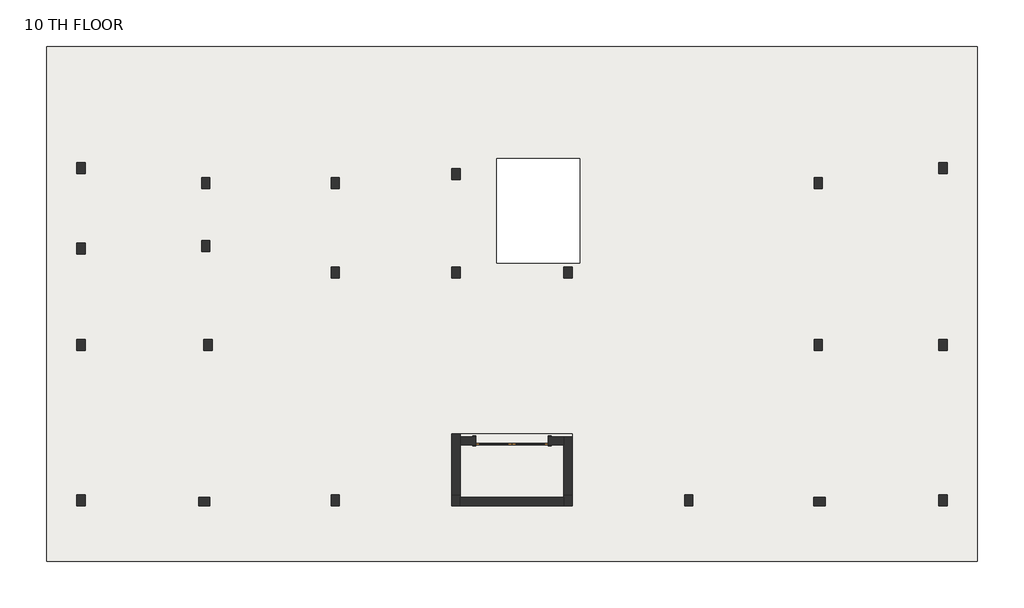
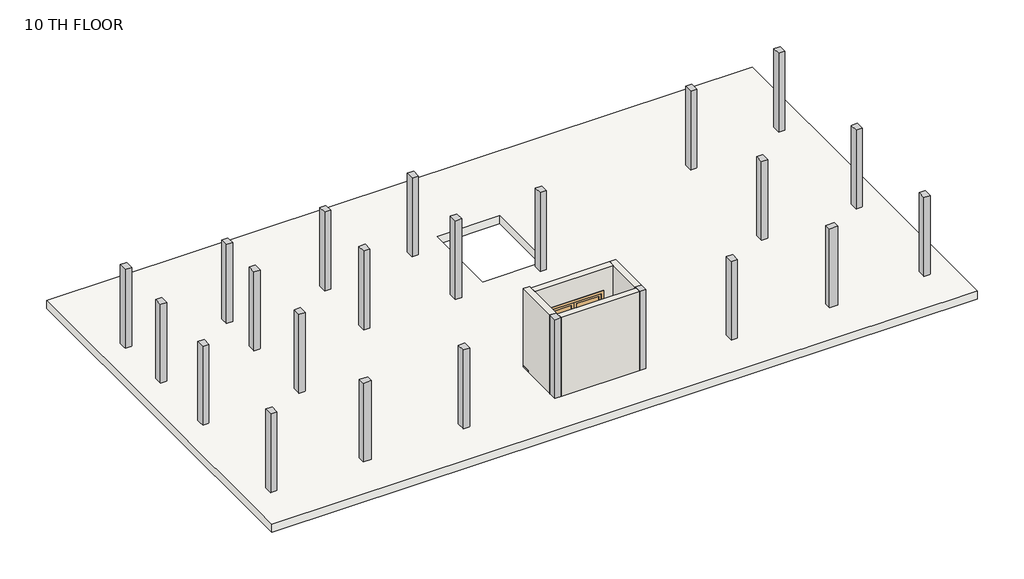
# One storey: 23 columns, 4 walls, 2 slabs, 1 door.
"""IFC4 building model written with IfcOpenShell, lengths in millimetres."""

from ifc_helpers import new_model, si_unit, frame, origin, place, context, project, spatial, polyline, outline, extrude, faceted_brep, transform, mapped, element, save
from components import column_69e4a381, door_77e2dd85

model = new_model("IFC4")

# Units and contexts
model_context = context("Model", 3, world=origin())
ifc_project = project(units=[si_unit("LENGTHUNIT", "METRE", prefix="MILLI")], contexts=[model_context])

# Site, building, storey
site = spatial("IfcSite", under=ifc_project)
building = spatial("IfcBuilding", under=site)
storey = spatial("IfcBuildingStorey", under=building, Name="10 TH FLOOR", Elevation=35204.4)

# Columns
placement = place(None, origin())
element("IfcColumn", 1, ObjectType="Rectangular Column : 1'X 9\"", at=placement, inside=storey, context=model_context, shape_type="SweptSolid", body=[
    extrude(outline(polyline([(-12224.6987957, -3709.2932671), (-12224.6987957, -4014.0932671), (-12453.2987957, -4014.0932671), (-12453.2987957, -3709.2932671), (-12224.6987957, -3709.2932671)])), frame((0.0, 0.0, 35204.4), z_axis=(0.0, 0.0, 1.0), x_axis=(1.0, 0.0, 0.0)), (0.0, 0.0, 1.0), 3048.0),
])
element("IfcColumn", 2, ObjectType="Rectangular Column : 1'X 9\"", at=placement, inside=storey, context=model_context, shape_type="SweptSolid", body=[
    extrude(outline(polyline([(-12224.6987957, 583.3067334), (-12224.6987957, 278.5067334), (-12453.2987957, 278.5067334), (-12453.2987957, 583.3067334), (-12224.6987957, 583.3067334)])), frame((0.0, 0.0, 35204.4), z_axis=(0.0, 0.0, 1.0), x_axis=(1.0, 0.0, 0.0)), (0.0, 0.0, 1.0), 3048.0),
])
element("IfcColumn", 3, ObjectType="Rectangular Column : 1'X 9\"", at=placement, inside=storey, context=model_context, shape_type="SweptSolid", body=[
    extrude(outline(polyline([(-12224.6987957, 3256.6567332), (-12224.6987957, 2951.8567332), (-12453.2987957, 2951.8567332), (-12453.2987957, 3256.6567332), (-12224.6987957, 3256.6567332)])), frame((0.0, 0.0, 35204.4), z_axis=(0.0, 0.0, 1.0), x_axis=(1.0, 0.0, 0.0)), (0.0, 0.0, 1.0), 3048.0),
])
element("IfcColumn", 4, ObjectType="Rectangular Column : 1'X 9\"", at=placement, inside=storey, context=model_context, shape_type="SweptSolid", body=[
    extrude(outline(polyline([(-8770.2987992, 5066.406733), (-8770.2987992, 4761.606733), (-8998.8987992, 4761.606733), (-8998.8987992, 5066.406733), (-8770.2987992, 5066.406733)])), frame((0.0, 0.0, 35204.4), z_axis=(0.0, 0.0, 1.0), x_axis=(1.0, 0.0, 0.0)), (0.0, 0.0, 1.0), 3048.0),
])
element("IfcColumn", 5, ObjectType="Rectangular Column : 1'X 9\"", at=placement, inside=storey, context=model_context, shape_type="SweptSolid", body=[
    extrude(outline(polyline([(-8770.2987992, 3326.5067332), (-8770.2987992, 3021.7067332), (-8998.8987992, 3021.7067332), (-8998.8987992, 3326.5067332), (-8770.2987992, 3326.5067332)])), frame((0.0, 0.0, 35204.4), z_axis=(0.0, 0.0, 1.0), x_axis=(1.0, 0.0, 0.0)), (0.0, 0.0, 1.0), 3048.0),
])
element("IfcColumn", 6, ObjectType="Rectangular Column : 1'X 9\"", at=placement, inside=storey, context=model_context, shape_type="SweptSolid", body=[
    extrude(outline(polyline([(-8713.148796, 583.3067334), (-8713.148796, 278.5067334), (-8941.748796, 278.5067334), (-8941.748796, 583.3067334), (-8713.148796, 583.3067334)])), frame((0.0, 0.0, 35204.4), z_axis=(0.0, 0.0, 1.0), x_axis=(1.0, 0.0, 0.0)), (0.0, 0.0, 1.0), 3048.0),
])
element("IfcColumn", 7, ObjectType="Rectangular Column : 1'X 9\"", at=placement, inside=storey, context=model_context, shape_type="SweptSolid", body=[
    extrude(outline(polyline([(-5188.8987995, 5066.406733), (-5188.8987995, 4761.606733), (-5417.4987995, 4761.606733), (-5417.4987995, 5066.406733), (-5188.8987995, 5066.406733)])), frame((0.0, 0.0, 35204.4), z_axis=(0.0, 0.0, 1.0), x_axis=(1.0, 0.0, 0.0)), (0.0, 0.0, 1.0), 3048.0),
])
element("IfcColumn", 8, ObjectType="Rectangular Column : 1'X 9\"", at=placement, inside=storey, context=model_context, shape_type="SweptSolid", body=[
    extrude(outline(polyline([(-5188.8987995, 2589.9067802), (-5188.8987995, 2285.1067802), (-5417.4987995, 2285.1067802), (-5417.4987995, 2589.9067802), (-5188.8987995, 2589.9067802)])), frame((0.0, 0.0, 35204.4), z_axis=(0.0, 0.0, 1.0), x_axis=(1.0, 0.0, 0.0)), (0.0, 0.0, 1.0), 3048.0),
])
element("IfcColumn", 9, ObjectType="Rectangular Column : 1'X 9\"", at=placement, inside=storey, context=model_context, shape_type="SweptSolid", body=[
    extrude(outline(polyline([(-5188.8987963, -3709.2932193), (-5188.8987963, -4014.0932193), (-5417.4987963, -4014.0932193), (-5417.4987963, -3709.2932193), (-5188.8987963, -3709.2932193)])), frame((0.0, 0.0, 35204.4), z_axis=(0.0, 0.0, 1.0), x_axis=(1.0, 0.0, 0.0)), (0.0, 0.0, 1.0), 3048.0),
])
element("IfcColumn", 10, ObjectType="Rectangular Column : 1'X 9\"", at=placement, inside=storey, context=model_context, shape_type="Brep", body=[
    faceted_brep([(1250.0012085, -3709.2932193, 35204.4), (1250.0012085, -4014.0932193, 35204.4), (1021.4012085, -4014.0932193, 35204.4), (1021.4012085, -3785.4932663, 35204.4), (1021.4012085, -3709.2932193, 35204.4), (1250.0012085, -3709.2932193, 38252.4), (1250.0012085, -4014.0932193, 38252.4), (1021.4012085, -4014.0932193, 38252.4), (1021.4012085, -3785.4932663, 38252.4), (1021.4012085, -3709.2932193, 38252.4)], [[[0, 1, 2, 3, 4]], [[5, 6, 1, 0]], [[6, 7, 2, 1]], [[7, 8, 9, 4, 3, 2]], [[9, 5, 0, 4]], [[5, 9, 8, 7, 6]]]),
])
element("IfcColumn", 11, ObjectType="Rectangular Column : 1'X 9\"", at=placement, inside=storey, context=model_context, shape_type="SweptSolid", body=[
    extrude(outline(polyline([(4590.1012082, -3709.2932193), (4590.1012082, -4014.0932193), (4361.5012082, -4014.0932193), (4361.5012082, -3709.2932193), (4590.1012082, -3709.2932193)])), frame((0.0, 0.0, 35204.4), z_axis=(0.0, 0.0, 1.0), x_axis=(1.0, 0.0, 0.0)), (0.0, 0.0, 1.0), 3048.0),
])
element("IfcColumn", 12, ObjectType="Rectangular Column : 1'X 9\"", at=placement, inside=storey, context=model_context, shape_type="SweptSolid", body=[
    extrude(outline(polyline([(11625.9012075, -3709.2932671), (11625.9012075, -4014.0932671), (11397.3012075, -4014.0932671), (11397.3012075, -3709.2932671), (11625.9012075, -3709.2932671)])), frame((0.0, 0.0, 35204.4), z_axis=(0.0, 0.0, 1.0), x_axis=(1.0, 0.0, 0.0)), (0.0, 0.0, 1.0), 3048.0),
])
element("IfcColumn", 13, ObjectType="Rectangular Column : 1'X 9\"", at=placement, inside=storey, context=model_context, shape_type="SweptSolid", body=[
    extrude(outline(polyline([(11625.9012075, 583.3067295), (11625.9012075, 278.5067295), (11397.3012075, 278.5067295), (11397.3012075, 583.3067295), (11625.9012075, 583.3067295)])), frame((0.0, 0.0, 35204.4), z_axis=(0.0, 0.0, 1.0), x_axis=(1.0, 0.0, 0.0)), (0.0, 0.0, 1.0), 3048.0),
])
element("IfcColumn", 14, ObjectType="Rectangular Column : 1'X 9\"", at=placement, inside=storey, context=model_context, shape_type="SweptSolid", body=[
    extrude(outline(polyline([(11625.9012075, 5479.1567329), (11625.9012075, 5174.3567329), (11397.3012075, 5174.3567329), (11397.3012075, 5479.1567329), (11625.9012075, 5479.1567329)])), frame((0.0, 0.0, 35204.4), z_axis=(0.0, 0.0, 1.0), x_axis=(1.0, 0.0, 0.0)), (0.0, 0.0, 1.0), 3048.0),
])
element("IfcColumn", 15, ObjectType="Rectangular Column : 1'X 9\"", at=placement, inside=storey, context=model_context, shape_type="SweptSolid", body=[
    extrude(outline(polyline([(8172.5040565, 5065.4824989), (8172.5040565, 4760.6824989), (7943.9040565, 4760.6824989), (7943.9040565, 5065.4824989), (8172.5040565, 5065.4824989)])), frame((0.0, 0.0, 35204.4), z_axis=(0.0, 0.0, 1.0), x_axis=(1.0, 0.0, 0.0)), (0.0, 0.0, 1.0), 3048.0),
])
element("IfcColumn", 16, ObjectType="Rectangular Column : 1'X 9\"", at=placement, inside=storey, context=model_context, shape_type="SweptSolid", body=[
    extrude(outline(polyline([(8171.5012047, 583.3067334), (8171.5012047, 278.5067334), (7942.9012047, 278.5067334), (7942.9012047, 583.3067334), (8171.5012047, 583.3067334)])), frame((0.0, 0.0, 35204.4), z_axis=(0.0, 0.0, 1.0), x_axis=(1.0, 0.0, 0.0)), (0.0, 0.0, 1.0), 3048.0),
])
element("IfcColumn", 17, ObjectType="Rectangular Column : 1'X 9\"", at=placement, inside=storey, context=model_context, shape_type="SweptSolid", body=[
    extrude(outline(polyline([(-9076.550543, -3785.4932196), (-8771.750543, -3785.4932196), (-8771.750543, -4014.0932196), (-9076.550543, -4014.0932196), (-9076.550543, -3785.4932196)])), frame((0.0, 0.0, 35204.4), z_axis=(0.0, 0.0, 1.0), x_axis=(1.0, 0.0, 0.0)), (0.0, 0.0, 1.0), 3048.0),
])
element("IfcColumn", 18, ObjectType="Rectangular Column : 1'X 9\"", at=placement, inside=storey, context=model_context, shape_type="SweptSolid", body=[
    extrude(outline(polyline([(-12453.2987957, 5174.3567339), (-12453.2987957, 5479.1567339), (-12224.6987957, 5479.1567339), (-12224.6987957, 5174.3567339), (-12453.2987957, 5174.3567339)])), frame((0.0, 0.0, 35204.4), z_axis=(0.0, 0.0, 1.0), x_axis=(1.0, 0.0, 0.0)), (0.0, 0.0, 1.0), 3048.0),
])
element("IfcColumn", 19, ObjectType="Rectangular Column : 1'X 9\"", at=placement, inside=storey, context=model_context, shape_type="SweptSolid", body=[
    extrude(outline(polyline([(-1845.5417538, 5320.4067329), (-1845.5417538, 5015.6067329), (-2074.1417538, 5015.6067329), (-2074.1417538, 5320.4067329), (-1845.5417538, 5320.4067329)])), frame((0.0, 0.0, 35204.4), z_axis=(0.0, 0.0, 1.0), x_axis=(1.0, 0.0, 0.0)), (0.0, 0.0, 1.0), 3048.0),
])
element("IfcColumn", 20, ObjectType="Rectangular Column : 1'X 9\"", at=placement, inside=storey, context=model_context, shape_type="SweptSolid", body=[
    extrude(outline(polyline([(-1845.5417538, 2589.906774), (-1845.5417538, 2285.106774), (-2074.1417538, 2285.106774), (-2074.1417538, 2589.906774), (-1845.5417538, 2589.906774)])), frame((0.0, 0.0, 35204.4), z_axis=(0.0, 0.0, 1.0), x_axis=(1.0, 0.0, 0.0)), (0.0, 0.0, 1.0), 3048.0),
])
element("IfcColumn", 21, ObjectType="Rectangular Column : 1'X 9\"", at=placement, inside=storey, context=model_context, shape_type="SweptSolid", body=[
    extrude(outline(polyline([(1253.2582462, 2589.9067742), (1253.2582462, 2285.1067742), (1024.6582462, 2285.1067742), (1024.6582462, 2589.9067742), (1253.2582462, 2589.9067742)])), frame((0.0, 0.0, 35204.4), z_axis=(0.0, 0.0, 1.0), x_axis=(1.0, 0.0, 0.0)), (0.0, 0.0, 1.0), 3048.0),
])
element("IfcColumn", 22, ObjectType="Rectangular Column : 1'X 9\"", at=placement, inside=storey, context=model_context, shape_type="Brep", body=[
    faceted_brep([(-1848.7987998, -3709.2932663, 35204.4), (-1848.7987998, -3785.4932663, 35204.4), (-1848.7987998, -4014.0932663, 35204.4), (-2077.3987998, -4014.0932663, 35204.4), (-2077.3987998, -3709.2932663, 35204.4), (-1848.7987998, -3709.2932663, 38252.4), (-1848.7987998, -3785.4932663, 38252.4), (-1848.7987998, -4014.0932663, 38252.4), (-2077.3987998, -4014.0932663, 38252.4), (-2077.3987998, -3709.2932663, 38252.4)], [[[0, 1, 2, 3, 4]], [[5, 6, 7, 2, 1, 0]], [[7, 8, 3, 2]], [[8, 9, 4, 3]], [[9, 5, 0, 4]], [[5, 9, 8, 7, 6]]]),
])
column_shape = column_69e4a381(model_context)
element("IfcColumn", 23, ObjectType="Rectangular Column : 1'X 9\"", at=placement, inside=storey, context=model_context, shape_type="MappedRepresentation", body=[
    mapped(column_shape, transform((8094.1646942, -3901.6914801, 0.0), x_axis=(0.0, 1.0, 0.0), y_axis=(-1.0, 0.0, 0.0), z_axis=(0.0, 0.0, 1.0))),
])

# Door
door_shape = door_77e2dd85(model_context)
element("IfcDoor", 24, ObjectType="M_Door-Double-Glass : 6'7\"X7'", at=placement, inside=storey, context=model_context, shape_type="MappedRepresentation", body=[
    mapped(door_shape, transform((-413.6987957, -2221.0120163, 35204.4), x_axis=(-1.0, 0.0, 0.0), y_axis=(0.0, -1.0, 0.0), z_axis=(0.0, 0.0, 1.0))),
])

# Slabs
element("IfcSlab", 25, ObjectType="Generic - 12\"", at=placement, inside=storey, context=model_context, shape_type="SweptSolid", body=[
    extrude(outline(polyline([(12464.1012075, 8698.6067329), (12464.1012075, -5550.7932662), (-13291.4987957, -5550.7932662), (-13291.4987957, 8698.6067329), (12464.1012075, 8698.6067329)]), holes=[polyline([(1456.6270108, 2700.0220048), (1456.6270108, 5595.6220048), (-829.3729892, 5595.6220048), (-829.3729892, 2700.0220048), (1456.6270108, 2700.0220048)])]), frame((0.0, 0.0, 34899.6), z_axis=(0.0, 0.0, 1.0), x_axis=(1.0, 0.0, 0.0)), (0.0, 0.0, 1.0), 304.8),
])
element("IfcSlab", 26, ObjectType="Generic - 12\"", at=placement, inside=storey, context=model_context, shape_type="SweptSolid", body=[
    extrude(outline(polyline([(1250.0012085, -2032.8932663), (1250.0012085, -2337.6932663), (-2077.3987998, -2337.6932663), (-2077.3987998, -2032.8932663), (1250.0012085, -2032.8932663)])), frame((0.0, 0.0, 34975.8), z_axis=(0.0, 0.0, 1.0), x_axis=(1.0, 0.0, 0.0)), (0.0, 0.0, 1.0), 304.8),
])

# Walls
element("IfcWall", 27, ObjectType="9\"", at=placement, inside=storey, context=model_context, shape_type="Brep", body=[
    faceted_brep([(-1848.7987998, -3709.2932663, 35204.4), (-1848.7987998, -2337.6932663, 35204.4), (-1848.7987998, -2109.0932663, 35204.4), (-1848.7987998, -2032.8932663, 35204.4), (-1848.7987998, -2032.8932663, 38252.4), (-1848.7987998, -2109.0932663, 38252.4), (-1848.7987998, -2337.6932663, 38252.4), (-1848.7987998, -3709.2932663, 38252.4), (-2077.3987998, -3709.2932663, 35204.4), (-2077.3987998, -3709.2932663, 38252.4), (-2077.3987998, -2032.8932663, 38252.4), (-2077.3987998, -2032.8932663, 35204.4)], [[[0, 1, 2, 3, 4, 5, 6, 7]], [[8, 9, 10, 11]], [[3, 2, 1, 0, 8, 11]], [[4, 3, 11, 10]], [[7, 6, 5, 4, 10, 9]], [[0, 7, 9, 8]]]),
])
element("IfcWall", 28, ObjectType="9\"", at=placement, inside=storey, context=model_context, shape_type="SweptSolid", body=[
    extrude(outline(polyline([(35204.4, -1848.7987998), (35204.4, -1416.9987957), (37338.0, -1416.9987957), (37338.0, 589.6012043), (35204.4, 589.6012043), (35204.4, 1021.4012085), (38252.4, 1021.4012085), (38252.4, -1848.7987998), (35204.4, -1848.7987998)])), frame((0.0, -2337.6932663, 0.0), z_axis=(0.0, 1.0, 0.0), x_axis=(0.0, 0.0, 1.0)), (0.0, 0.0, 1.0), 228.6),
])
element("IfcWall", 29, ObjectType="9\"", at=placement, inside=storey, context=model_context, shape_type="Brep", body=[
    faceted_brep([(1021.4012085, -2109.0932663, 35204.4), (1021.4012085, -2337.6932663, 35204.4), (1021.4012085, -3709.2932193, 35204.4), (1021.4012085, -3709.2932193, 38252.4), (1021.4012085, -2337.6932663, 38252.4), (1021.4012085, -2109.0932663, 38252.4), (1250.0012085, -2109.0932663, 35204.4), (1250.0012085, -2109.0932663, 38252.4), (1250.0012085, -3709.2932193, 38252.4), (1250.0012085, -3709.2932193, 35204.4)], [[[0, 1, 2, 3, 4, 5]], [[6, 7, 8, 9]], [[2, 1, 0, 6, 9]], [[3, 2, 9, 8]], [[5, 4, 3, 8, 7]], [[0, 5, 7, 6]]]),
])
element("IfcWall", 30, ObjectType="9\"", at=placement, inside=storey, context=model_context, shape_type="SweptSolid", body=[
    extrude(outline(polyline([(1021.4012085, -4014.0932663), (-1848.7987998, -4014.0932663), (-1848.7987998, -3785.4932663), (1021.4012085, -3785.4932663), (1021.4012085, -4014.0932663)])), frame((0.0, 0.0, 35204.4), z_axis=(0.0, 0.0, 1.0), x_axis=(1.0, 0.0, 0.0)), (0.0, 0.0, 1.0), 3048.0),
])

save(model, "model.ifc")

# Revit data of these elements
# Type "Rectangular Column : 1'X 9\""
#   Assembly Code = "B1010200"
#   Depth = 1' - 0"
#   Offset Base = 0' - 0"
#   Offset Top = 0' - 0"
#   Width = 0' - 9"
#   Material = none
# Type "M_Door-Double-Glass : 6'7\"X7'"
#   Type Mark = "16"
#   Construction Type Id = "opn-d45"
#   Assembly Code = "C1020"
#   Analytic Construction = "Wood frame, double glass door "
#   W = 3' - 3 1/2"
#   Thickness = 0' - 1.9685"
#   Thermal Resistance (R) = 1.8150 (h·ft²·°F)/BTU
#   Swing Angle [instance default] = 90.00°
#   Heat Transfer Coefficient (U) = 0.5510 BTU/(h·ft²·°F)
#   Height = 7' - 0"
#   Bottom Rail = 0' - 3.93701"
#   Top Rail = 0' - 3.93701"
#   Stiles = 0' - 3.93701"
#   Trim Projection = 0' - 0.98425"
#   Trim Width = 0' - 3.14961"
#   Width = 6' - 7"
#   Define Thermal Properties by = 1
#   Glazing = Glass
#   Panel Material = Wood - Birch - Solid Stained Light Low Gloss
#   Trim Material = Paint - Sienna
#   Visual Light Transmittance = 0
#   Solar Heat Gain Coefficient = 0
#   Function = (empty or 0)
#   Wall Closure = (empty or 0)
# Type "Generic - 12\""
#   Assembly Code = "B1010"
#   Function = 0
#   Layers, outside or top first: 1' - 0" no material (function 1)
# Type "9\""
#   Assembly Code = "B2010"
#   Layers, outside or top first: 0' - 9" no material (function 1)
# Elements 1, 2, 3, 4, 5, 6, 7, 8, 9, 11, 12, 13, 14, 15, 16, 17, 18, 19, 20, 21, 23 (IfcColumn, "Rectangular Column : 1'X 9\"")
#   Phase Created = New Construction
# Elements 10, 22 (IfcColumn, "Rectangular Column : 1'X 9\"")
#   Phase Created = New Construction
#   Materials on its faces: "Default Wall"
# Element 24 (IfcDoor, "M_Door-Double-Glass : 6'7\"X7'")
#   Swing Angle = 90.00°
#   Phase Created = New Construction
#   Materials on its faces: "Wood - Birch - Solid Stained Light Low Gloss", "Paint - Sienna", "Glass"
# Element 25 (IfcSlab, "Generic - 12\"")
#   Height Offset From Level = 0' - 0"
#   Phase Created = New Construction
#   Materials on its faces: "Default Floor"
# Element 26 (IfcSlab, "Generic - 12\"")
#   Height Offset From Level = 0' - 3"
#   Phase Created = New Construction
#   Materials on its faces: "Default Floor"
# Elements 27, 28, 29, 30 (IfcWall, "9\"")
#   Top Offset = 0' - 0"
#   Base Offset = 0' - 0"
#   wall height = 10' - 0"
#   Phase Created = New Construction
#   Base Constraint = 10 TH FLOOR
#   Top Constraint = ROOF
#   Materials on its faces: "Default Wall"
# Materials
#   "Glass": class "Glass", colour RGB 0 128 192, transparency 0.75, Description = "Soda Lime Glass", Cost = 0
#   "Wood - Birch - Solid Stained Light Low Gloss": class "Wood", colour RGB 210 159 95, transparency 0, Cost = 0
#   "Paint - Sienna": colour RGB 118 70 51, transparency 0, Cost = 0
#   "Default Wall": colour RGB 128 128 128, transparency 0, Cost = 0
#   "Default Floor": colour RGB 128 128 128, transparency 0, Cost = 0
